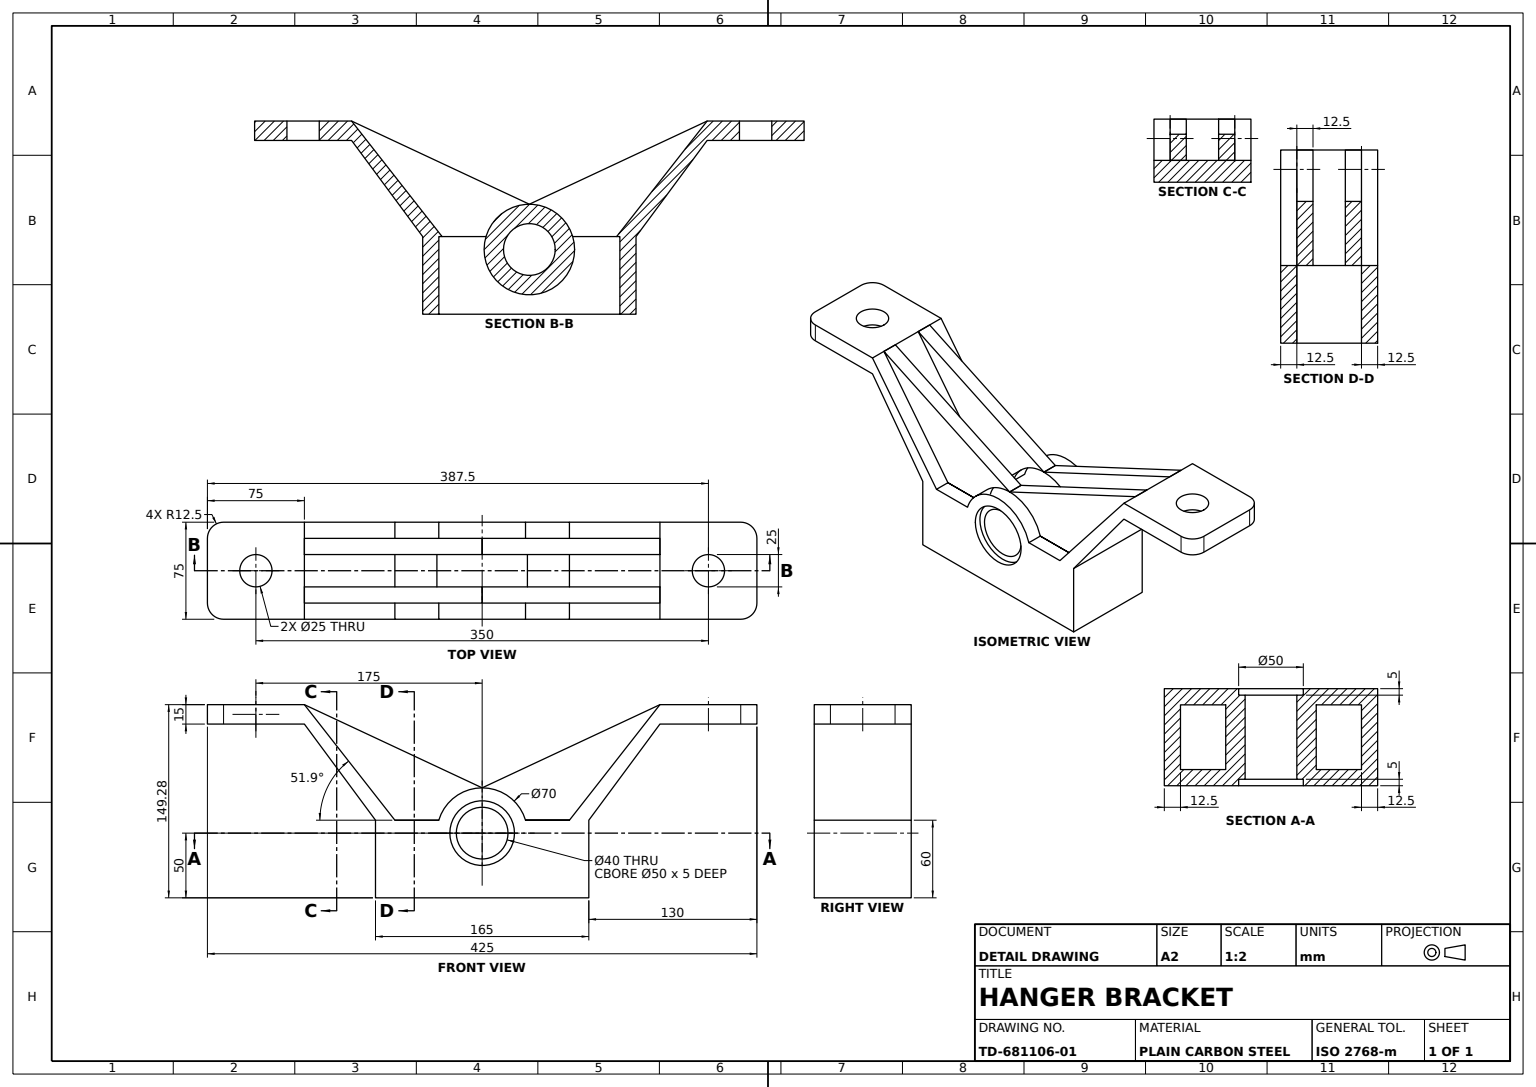
SolidWorks part; units mm, degrees
material "Plain Carbon Steel"
ref_plane "Front Plane" through (0, 0, 0) normal (0, 0, 1) x (1, 0, 0)
ref_plane "Top Plane" through (0, 0, 0) normal (0, 1, 0) x (1, 0, 0)
ref_plane "Right Plane" through (0, 0, 0) normal (1, 0, 0) x (0, 0, -1)
sketch "Bracket Profile Sketch" plane through (0, 0, 0) normal (0, 1, 0) x (1, 0, 0)
  line L1 (82.5, 0) -> (82.5, 37.5)
  line L2 (82.5, 37.5) -> (-82.5, 37.5)
  line L3 (-82.5, 37.5) -> (-82.5, -37.5)
  line L4 (-82.5, -37.5) -> (82.5, -37.5)
  line L5 (82.5, -37.5) -> (82.5, 0)
  dimension "D1" = 165
  dimension "D2" = 75
  dimension "D3" = 82.5
extrude "Bracket Body Thin 60x12.5" add sketch "Bracket Profile Sketch" along normal blind 60 thin thin type one direction reverse wall 12.5
sketch "Flange Pads Sketch" plane through (0, 0, 37.5) normal (0, 0, 1) x (1, 0, 0)
  line L0 (82.5, 60) -> (82.5, 0) construction
  line L1 (82.5, 60) -> (67.5, 60)
  line L2 (-137.5, 149.281) -> (-67.5, 60)
  line L5 (-137.5, 149.281) -> (-212.5, 149.281)
  line L6 (-212.5, 149.281) -> (-212.5, 134.281)
  line L7 (-82.5, 60) -> (-67.5, 60)
  line L8 (-82.5, 60) -> (82.5, 60) construction
  line L12 (-212.5, 134.281) -> (-137.5, 134.281)
  line L13 (-137.5, 134.281) -> (-82.5, 60)
  line L14 (137.5, 149.281) -> (67.5, 60)
  line L15 (137.5, 134.281) -> (82.5, 60)
  line L16 (212.5, 134.281) -> (137.5, 134.281)
  line L17 (212.5, 149.281) -> (212.5, 134.281)
  line L18 (137.5, 149.281) -> (212.5, 149.281)
  line L19 (-82.5, 0) -> (82.5, 0) construction
  dimension "D1" = 55
  dimension "D2" = 130
  dimension "D3" = 15
  dimension "D4" = 150
  dimension "D5" = 134.281
extrude "Mounting Flange Pads" add sketch "Flange Pads Sketch" against normal blind 75
sketch "Flange Holes Sketch" plane through (0, 149.281, 0) normal (0, 1, 0) x (1, 0, 0)
  line L0 (212.5, 37.5) -> (212.5, -37.5) construction
  line L1 (212.5, -37.5) -> (137.5, -37.5) construction
  circle A0 centre (175, 0) radius 12.5
  circle A1 centre (-175, 0) radius 12.5
  dimension "D1" = 25
  dimension "D2" = 37.5
  dimension "D3" = 387.5
  dimension "D4" = 37.5
extrude "Flange Mounting Holes 2x" cut sketch "Flange Holes Sketch" against normal blind 75
fillet "Flange Corner Fillet R12.5 A" radius 12.5 2 edges at (212.5, 141.781, 37.5) (-212.5, 141.781, 37.5)
fillet "Flange Corner Fillet R12.5 B" radius 12.5 2 edges at (-212.5, 141.781, -37.5) (212.5, 141.781, -37.5)
sketch "Bearing Boss Sketch" plane through (0, 0, 37.5) normal (0, 0, 1) x (1, 0, 0)
  line L0 (200, 134.281) -> (200, 149.281) construction
  line L1 (200, 149.281) -> (137.5, 149.281) construction
  circle A0 centre (0, 50) radius 35
  dimension "D1" = 70
  dimension "D2" = 200
  dimension "D3" = 99.281
extrude "Bearing Boss" add sketch "Bearing Boss Sketch" against normal blind 75
sketch "Bore Recess A Sketch" plane through (0, 0, 37.5) normal (0, 0, 1) x (1, 0, 0)
  circle A0 centre (0, 50) radius 25
  dimension "D1" = 50
extrude "Bore Recess A 5mm" cut sketch "Bore Recess A Sketch" against normal blind 5
sketch "Bearing Bore Sketch" plane through (0, 0, 32.5) normal (0, 0, 1) x (1, 0, 0)
  circle A0 centre (0, 50) radius 20
  dimension "D1" = 40
extrude "Bearing Bore" cut sketch "Bearing Bore Sketch" against normal blind 109
sketch "Bore Recess B Sketch" plane through (0, 0, -37.5) normal (0, 0, -1) x (-1, 0, 0)
  circle A0 centre (0, 50) radius 25
  dimension "D1" = 50
extrude "Bore Recess B 5mm" cut sketch "Bore Recess B Sketch" against normal blind 5
ref_plane "Rib Plane" through (0, 0, 25) normal (0, 0, 1) x (1, 0, 0)
sketch "Rib Sketch" plane through (0, 0, 25) normal (0, 0, 1) x (1, 0, 0)
  line L0 (-137.5, 149.281) -> (0, 85)
  line L1 (-137.5, 149.281) -> (-67.5, 60)
  line L2 (-67.5, 60) -> (-33.541, 60)
  arc A0 (33.541, 60) -> (-33.541, 60) centre (0, 50) ccw construction
  arc A1 (-33.541, 60) -> (0, 85) centre (0, 50) cw
extrude "Rib" add sketch "Rib Sketch" against normal blind 12.5 separate body
mirror "Rib Mirror Front Plane" about plane through (0, 0, 0) normal (0, 0, 1) of bodies 108
mirror "Rib Mirror Right Plane" about plane through (0, 0, 0) normal (1, 0, 0) of bodies 109 108
